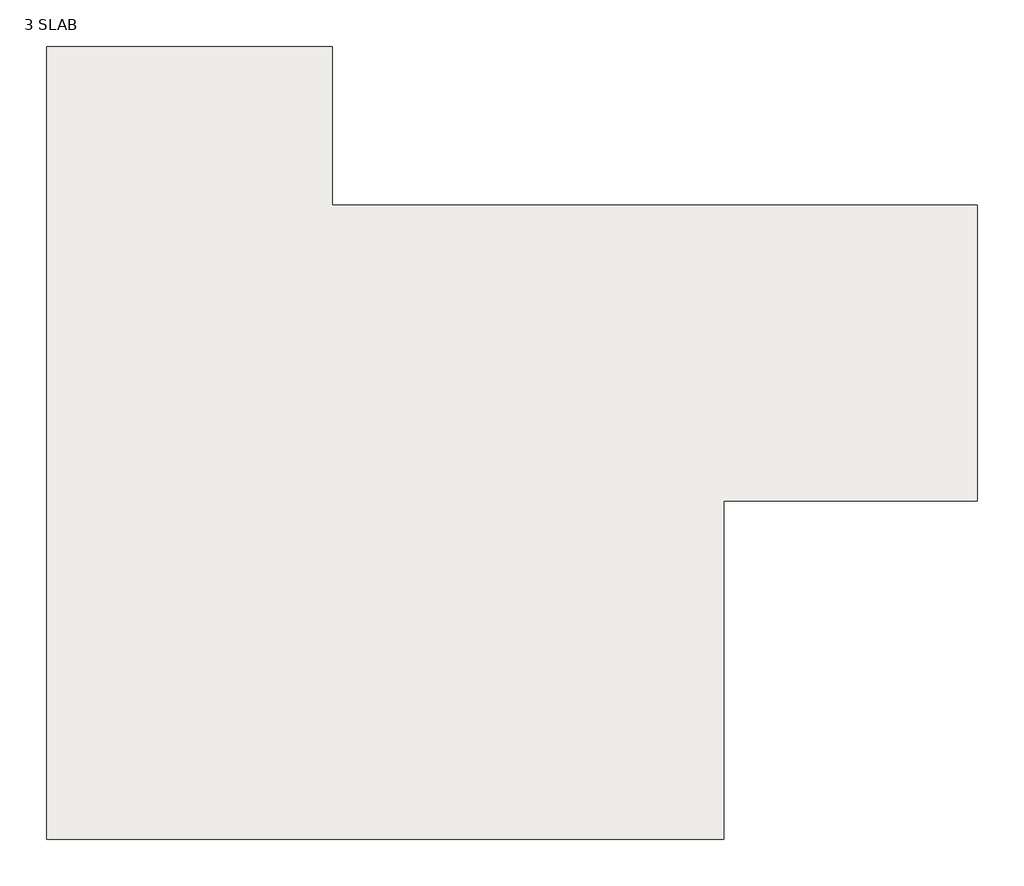
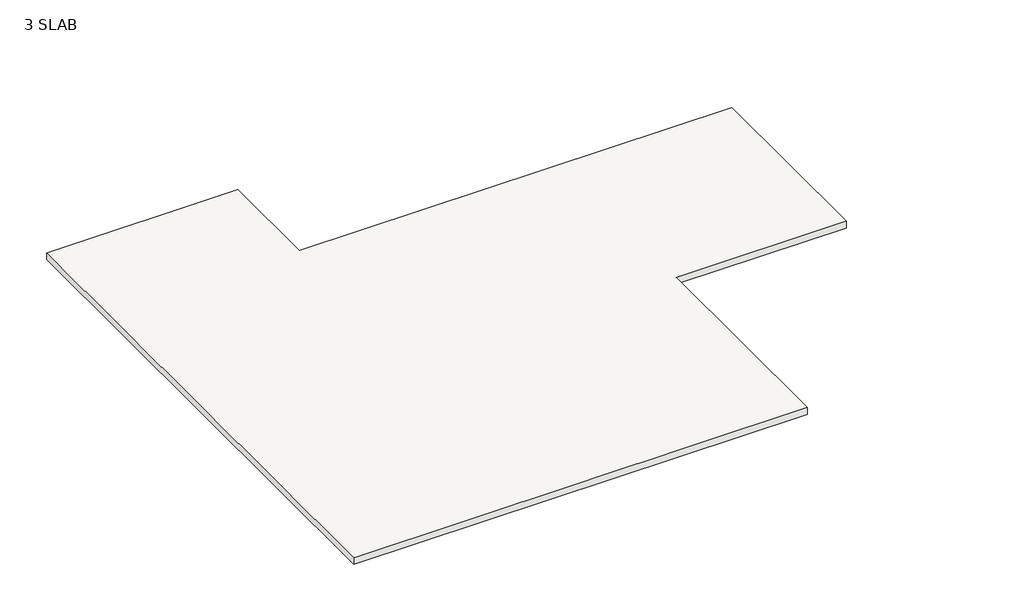
# One storey: 1 slab.
"""IFC4 building model written with IfcOpenShell, lengths in millimetres."""

from ifc_helpers import new_model, si_unit, frame, origin, place, context, project, spatial, polyline, outline, extrude, element, save

model = new_model("IFC4")

# Units and contexts
model_context = context("Model", 3, world=origin())
ifc_project = project(units=[si_unit("LENGTHUNIT", "METRE", prefix="MILLI")], contexts=[model_context])

# Site, building, storey
site = spatial("IfcSite", under=ifc_project)
building = spatial("IfcBuilding", under=site)
storey = spatial("IfcBuildingStorey", under=building, Name="3 SLAB", Elevation=3962.4)

# Slab
placement = place(None, origin())
element("IfcSlab", 1, ObjectType="6\"", at=placement, inside=storey, context=model_context, shape_type="SweptSolid", body=[
    extrude(outline(polyline([(-4260.6149535, 9951.3658196), (-145.8149535, 9951.3658196), (-145.8149535, 7665.3658196), (9150.5850465, 7665.3658196), (9150.5850465, 3398.1658196), (5492.9850465, 3398.1658196), (5492.9850465, -1478.6341804), (-4260.6149535, -1478.6341804), (-4260.6149535, 9951.3658196)])), frame((0.0, 0.0, 3810.0), z_axis=(0.0, 0.0, 1.0), x_axis=(1.0, 0.0, 0.0)), (0.0, 0.0, 1.0), 152.4),
])

save(model, "model.ifc")

# Revit data of these elements
# Type "6\""
#   Assembly Code = "B1010"
#   Function = 0
#   Layers, outside or top first: 0' - 6" no material (function 1)
# Element 1 (IfcSlab, "6\"")
#   built-in parameter 1001955 = 3.14159 (stored number, unit not read)
#   Height Offset From Level = 0' - 0"
#   Phase Created = New Construction
#   Materials on its faces: "Default Floor"
# Materials
#   "Default Floor": colour RGB 128 128 128, transparency 0, Cost = 0
